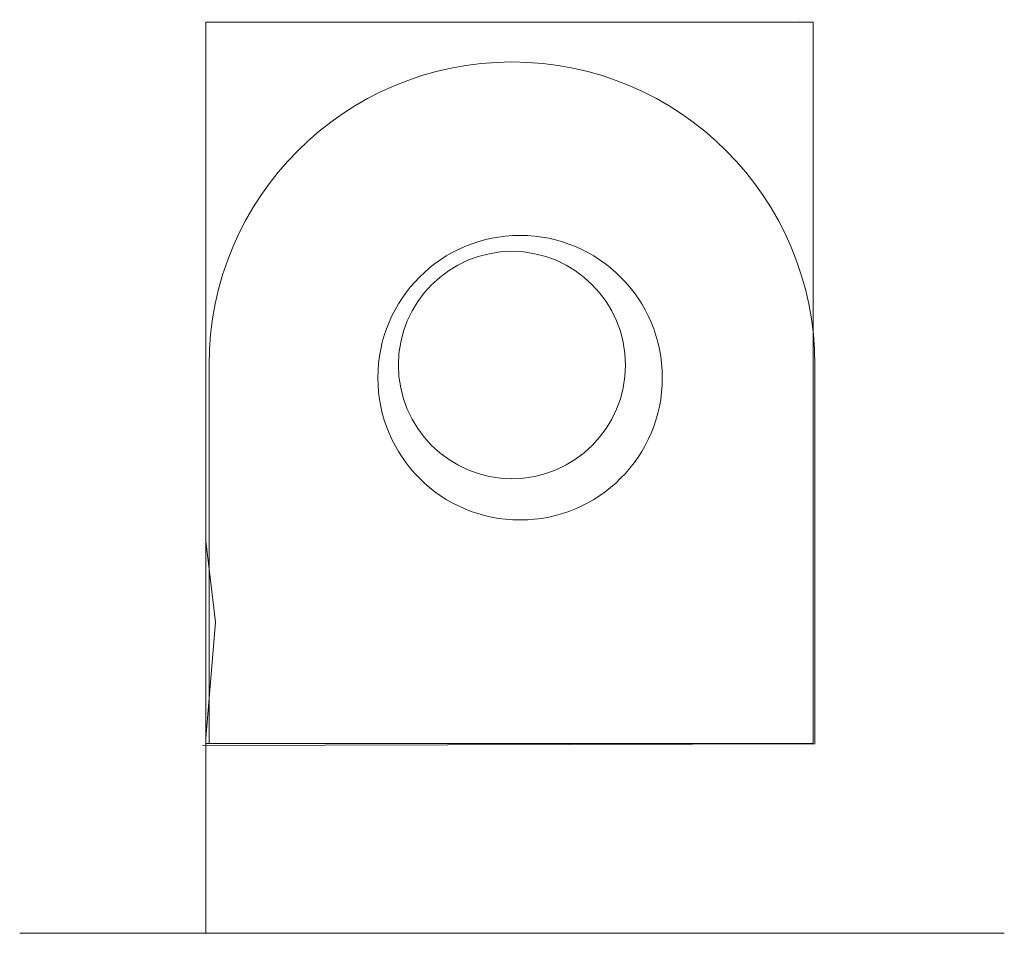
# Model space of a CAD drawing. Units: inches. Extents: x 42 to 172, y 0 to 121.
import ezdxf

# ---------------------------------------------------------------- set-up
doc = ezdxf.new("R2010")
doc.units = ezdxf.units.IN
doc.header["$MEASUREMENT"] = 0
doc.layers.add('M-CONS', color=8, linetype='Continuous', lineweight=13)

msp = doc.modelspace()

# ---------------------------------------------------------------- linework, layer by layer
at = {"layer": 'M-CONS'}
for p, q in [((145.06, 120.58, 99.57), (145.06, 120.58, 99.57)), ((146.9, 120.27, 199.57), (146.9, 120.07, 101.54)), ((146.9, 120.07, 101.54), (146.9, 120.07, 101.54)), ((146.9, 120.07, 199.32), (146.9, 119.53, 100.51)), ((147.13, 75, 99.71), (147.13, 60, 99.71)), ((147.13, 75, 99.71), (147.13, 40, 99.71)), ((67.13, 40, 99.71), (67.13, 55, 99.71)), ((147.13, 40, 99.71), (147.13, 55, 99.71)), ((147.13, 40, 99.71), (147.13, 40, 99.71)), ((107.13, 0, 9.71), (67.13, 0, 9.71)), ((147.13, 0, 9.71), (147.13, 0, 34.71))]:
    msp.add_line(p, q, dxfattribs=at)
at = {"layer": 'M-CONS', "extrusion": (0, 0, -1)}
for p, q in [((66.73, 51.75, 126.72), (67.99, 41.08, 133.24)), ((67.99, 41.08, 133.24), (66.73, 25.71, 119.38))]:
    msp.add_line(p, q, dxfattribs=at)
at = {"layer": 'M-CONS', "extrusion": (-1, 0, 0)}
for q in [(66.73, 25.07, 119.81), (66.73, 0, 99.57)]:
    msp.add_line((66.73, 25.07, 119.81), q, dxfattribs=at)
at = {"layer": 'M-CONS', "elevation": 99.57}
msp.add_lwpolyline([(66.73, 25.04), (146.9, 25.04), (146.9, 120.27), (66.73, 120.27)], close=True, dxfattribs=at)
at = {"layer": 'M-CONS', "elevation": 99.71}
msp.add_lwpolyline([(66.27, 24.79), (147.13, 25), (147.13, 75, 1), (67.13, 75), (67.13, 25)], format="xyb", dxfattribs=at)
at = {"layer": 'M-CONS', "extrusion": (-1, 0, 0), "elevation": -67.13}
msp.add_lwpolyline([(-25.37, 198.4), (-26.48, 198.4), (-26.48, 198.73), (-25.37, 198.73)], close=True, dxfattribs=at)
at = {"layer": 'M-CONS', "extrusion": (0, -1, 0)}
msp.add_lwpolyline([(42.13, 99.71), (172.13, 99.71), (172.13, 34.71, -0.414214), (147.13, 9.71), (67.13, 9.71, -0.414214), (42.13, 34.71)], format="xyb", close=True, dxfattribs=at)
at = {"layer": 'M-CONS'}
msp.add_lwpolyline([(172.13, 0), (172.13, 0), (172.13, 0), (172.13, 0)], close=True, dxfattribs=at)
at = {"layer": 'M-CONS', "extrusion": (0, 0, -1)}
msp.add_circle((-108.2, 73.33, -74.57), 18.78, dxfattribs=at)
at = {"layer": 'M-CONS'}
msp.add_circle((107.13, 75, 99.71), 15, dxfattribs=at)
at = {"layer": 'M-CONS', "extrusion": (0, -1, 0)}
for centre in [(67.13, 34.71), (147.13, 34.71)]:
    msp.add_circle(centre, 10, dxfattribs=at)

doc.saveas('drawing.dxf')
